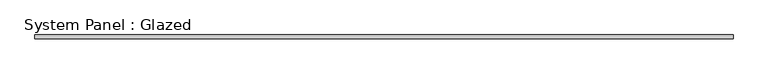
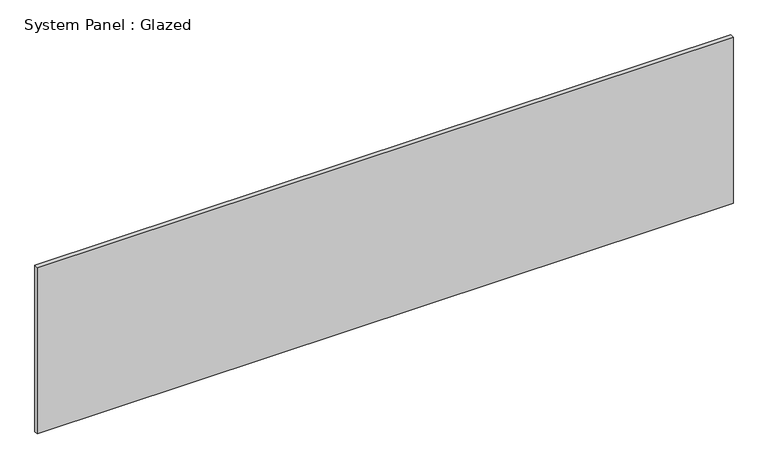
"""IFC4 building model written with IfcOpenShell, lengths in millimetres: plate geometry, System Panel : Glazed."""

from ifc_helpers import new_model, si_unit, origin, origin_with_axes, place, context, project, spatial, polyline, outline, extrude, source, transform, mapped, element, save


def system_panel_glazed_05863204(model_context):
    return source(origin(), model_context, "Body", "SweptSolid", [
        extrude(outline(polyline([(2288.8245158, 19.05), (-2288.8245158, 19.05), (-2288.8245158, 44.45), (2288.8245158, 44.45), (2288.8245158, 19.05)])), origin_with_axes(), (0.0, 0.0, 1.0), 1155.7),
    ])


if __name__ == "__main__":
    model = new_model("IFC4")
    model_context = context("Model", 3, world=origin())
    ifc_project = project(units=[si_unit("LENGTHUNIT", "METRE", prefix="MILLI")], contexts=[model_context])
    site = spatial("IfcSite", under=ifc_project)
    building = spatial("IfcBuilding", under=site)
    placement = place(None, origin())
    system_panel_glazed_shape = system_panel_glazed_05863204(model_context)
    element("IfcPlate", 1, ObjectType="System Panel : Glazed", at=placement, inside=building, context=model_context, shape_type="MappedRepresentation", body=[
        mapped(system_panel_glazed_shape, transform((0.0, 0.0, 0.0), x_axis=(1.0, 0.0, 0.0), y_axis=(0.0, 1.0, 0.0), z_axis=(0.0, 0.0, 1.0))),
    ])
    save(model, "model.ifc")

# Revit data of these elements
# Type "System Panel : Glazed"
#   Construction Type Id = "GSP4R"
#   Analytic Construction = "1/8 in Pilkington single glazing"
#   Visual Light Transmittance = 0.9
#   Solar Heat Gain Coefficient = 0.86
#   Heat Transfer Coefficient (U) = 1.18115 BTU/(h·ft²·°F)
# Element 1 (IfcPlate, "System Panel : Glazed")
#   Materials on its faces: "Glass"
# Materials
#   "Glass": class "Glass", colour RGB 0 128 192, transparency 0.75, Description = "Soda Lime Glass", Cost = 0
